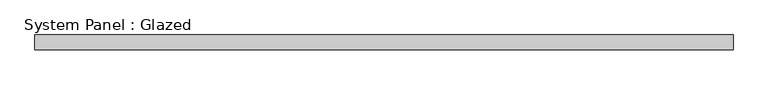
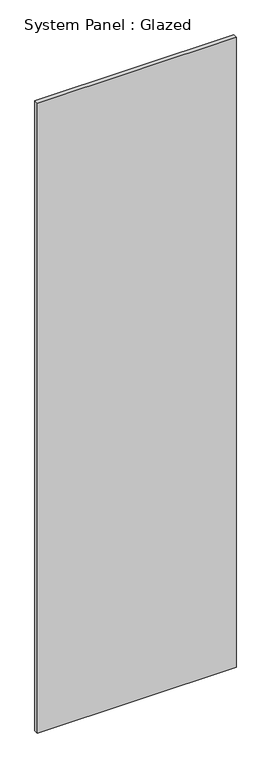
"""IFC4 building model written with IfcOpenShell, lengths in millimetres: plate geometry, System Panel : Glazed."""

from ifc_helpers import new_model, si_unit, origin, origin_with_axes, place, context, project, spatial, polyline, outline, extrude, source, transform, mapped, element, save


def system_panel_glazed_095a6893(model_context):
    return source(origin(), model_context, "Body", "SweptSolid", [
        extrude(outline(polyline([(596.9, 24.5), (-596.9, 24.5), (-596.9, 49.5), (596.9, 49.5), (596.9, 24.5)])), origin_with_axes(), (0.0, 0.0, 1.0), 4000.0),
    ])


if __name__ == "__main__":
    model = new_model("IFC4")
    model_context = context("Model", 3, world=origin())
    ifc_project = project(units=[si_unit("LENGTHUNIT", "METRE", prefix="MILLI")], contexts=[model_context])
    site = spatial("IfcSite", under=ifc_project)
    building = spatial("IfcBuilding", under=site)
    placement = place(None, origin())
    system_panel_glazed_shape = system_panel_glazed_095a6893(model_context)
    element("IfcPlate", 1, ObjectType="System Panel : Glazed", at=placement, inside=building, context=model_context, shape_type="MappedRepresentation", body=[
        mapped(system_panel_glazed_shape, transform((0.0, 0.0, 0.0), x_axis=(1.0, 0.0, 0.0), y_axis=(0.0, 1.0, 0.0), z_axis=(0.0, 0.0, 1.0))),
    ])
    save(model, "model.ifc")

# Revit data of these elements
# Type "System Panel : Glazed"
#   Keynote = "H11"
#   Construction Type Id = "GSP4R"
#   Analytic Construction = "1/8 in Pilkington single glazing"
#   Visual Light Transmittance = 0.9
#   Solar Heat Gain Coefficient = 0.86
#   Heat Transfer Coefficient (U) = 6.7069 W/(m²·K)
#   Define Thermal Properties by = 1
# Element 1 (IfcPlate, "System Panel : Glazed")
#   Materials on its faces: "Glass"
# Materials
#   "Glass": class "Glass", colour RGB 0 128 192, transparency 0.9, Description = "Soda Lime Glass", Cost = 0
